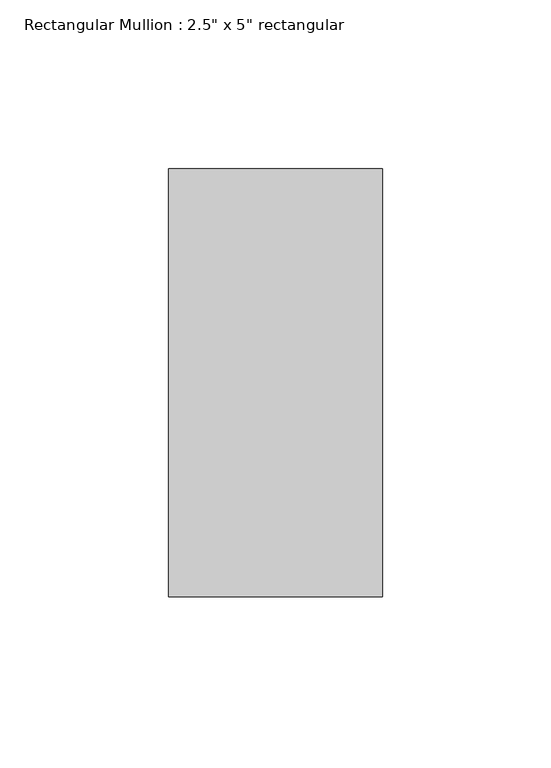
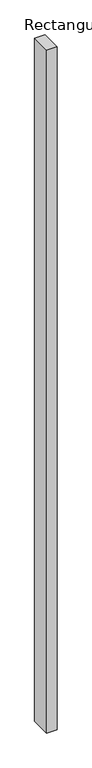
"""IFC4 building model written with IfcOpenShell, lengths in millimetres: member geometry."""

from ifc_helpers import new_model, si_unit, frame, origin, place, context, project, spatial, polyline, outline, extrude, source, transform, mapped, element, save


def member_8f078878(model_context):
    return source(origin(), model_context, "Body", "SweptSolid", [
        extrude(outline(polyline([(0.0, 63.5), (0.0, -63.5), (-63.5, -63.5), (-63.5, 63.5), (0.0, 63.5)])), frame((0.0, 0.0, -4396.5549749), z_axis=(0.0, 0.0, 1.0), x_axis=(1.0, 0.0, 0.0)), (0.0, 0.0, 1.0), 4396.5549749),
    ])


if __name__ == "__main__":
    model = new_model("IFC4")
    model_context = context("Model", 3, world=origin())
    ifc_project = project(units=[si_unit("LENGTHUNIT", "METRE", prefix="MILLI")], contexts=[model_context])
    site = spatial("IfcSite", under=ifc_project)
    building = spatial("IfcBuilding", under=site)
    placement = place(None, origin())
    member_shape = member_8f078878(model_context)
    element("IfcMember", 1, ObjectType="Rectangular Mullion : 2.5\" x 5\" rectangular", at=placement, inside=building, context=model_context, shape_type="MappedRepresentation", body=[
        mapped(member_shape, transform((0.0, 0.0, 0.0), x_axis=(1.0, 0.0, 0.0), y_axis=(0.0, 1.0, 0.0), z_axis=(0.0, 0.0, 1.0))),
    ])
    save(model, "model.ifc")

# Revit data of these elements
# Type "Rectangular Mullion : 2.5\" x 5\" rectangular"
#   built-in parameter 1007304 = 0.416667 (stored number, unit not read)
#   built-in parameter 1007301 = 0.104167 (stored number, unit not read)
#   built-in parameter 1007300 = 0.104167 (stored number, unit not read)
# Element 1 (IfcMember, "Rectangular Mullion : 2.5\" x 5\" rectangular")
#   Materials on its faces: "Iron, Ductile"
# Materials
#   "Iron, Ductile": class "Metal", colour RGB 0 0 0, transparency 0, Description = "Ductile cast iron", Cost = 0
